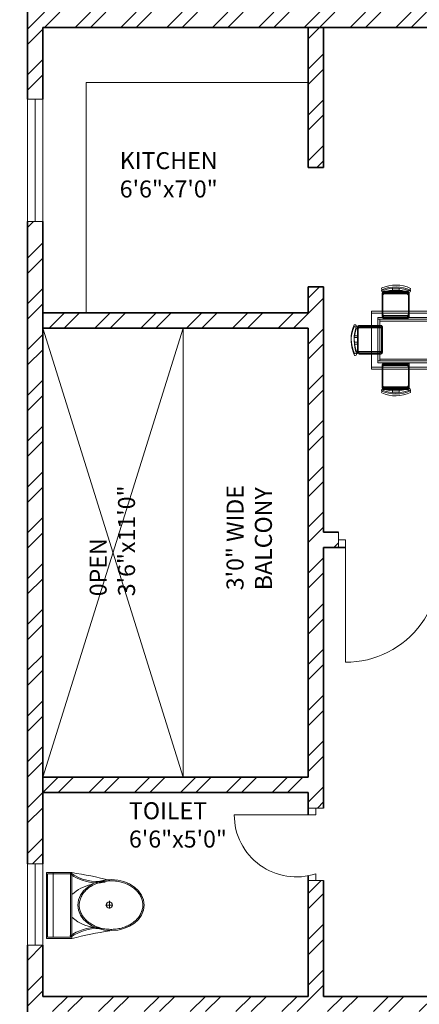
# Model space of a CAD drawing. Units: inches. Extents: x 2168 to 3056, y 1130 to 2629.
# Tile 4 of 42: x 2329 to 2447, y 1789 to 2079. Entities that reach past the tile are written whole.
import ezdxf

# ---------------------------------------------------------------- set-up
doc = ezdxf.new("R2010")
doc.units = ezdxf.units.IN
for name, color, linetype, lineweight in [('A-ANNO-DIMS', 2, 'Continuous', 18), ('A-AREA-IDEN', 7, 'Continuous', 18), ('A-DOOR', 21, 'Continuous', 18), ('A-FLOR-CASE', 71, 'Continuous', 18), ('A-FLOR-FIXT', 9, 'Continuous', 18), ('A-FLOR-OTLN', 7, 'Continuous', 18), ('A-FURN', 8, 'Continuous', 13), ('A-GLAZ', 201, 'Continuous', 18), ('A-WALL', 7, 'Continuous', 35)]:
    doc.layers.add(name, color=color, linetype=linetype, lineweight=lineweight)
doc.layers.add('A-WALL-PATT', color=143, linetype='Continuous', lineweight=13, true_color=0x7aafdf)
doc.styles.get("Standard").update_dxf_attribs({"font": 'arial.ttf'})
doc.dimstyles.get("Standard").update_dxf_attribs({"dimtxt": 0.18, "dimasz": 0.18, "dimexe": 0.18, "dimexo": 0.0625, "dimgap": 0.09, "dimtad": 0, "dimtih": 1, "dimtoh": 1, "dimdec": 4, "dimzin": 0, "dimdsep": 46, "dimtxsty": 'Standard', "dimcen": 0.09, "dimadec": 0, "dimazin": 0, "dimtfac": 1, "dimtdec": 4, "dimtofl": 0, "dimtmove": 0, "dimatfit": 3, "dimfxl": 1, "dimtolj": 1, "dimtzin": 0, "dimarcsym": 0})

# ---------------------------------------------------------------- blocks, each defined once
blk = doc.blocks.new('A$C31115884')
for p, q in [((283.1, 497.7), (223.4, 497.7)), ((257.5, 466.4), (257.5, 523.2)), ((0, 200), (0, 0)), ((520, 200), (0, 200)), ((10, 190), (10, 10)), ((510, 190), (10, 190)), ((510, 10), (510, 190)), ((520, 0), (520, 200)), ((510, 54.5), (0, 54.5)), ((10, 10), (510, 10)), ((0, 0), (520, 0))]:
    blk.add_line(p, q)
blk.add_circle((255.6, 496.4), 23.6)
for centre, radius, start, end in [((2777.7, -204.6), 2807, 165.4549, 171.71327), ((3237, 905), 2807, 188.28673, 194.5451), ((-294.5, 403.3), 364.7, 324.20913, 9.34987), ((-294.5, 403.3), 374.7, 324.20913, 9.34987), ((139.5, 406.2), 293.5, 315.84364, 2.65635), ((805.8, 403.3), 374.7, 179.20365, 215.79087), ((805.8, 403.3), 364.7, 170.65013, 215.79087), ((383.6, 406.2), 293.5, 190.27735, 224.15636)]:
    blk.add_arc(centre, radius, start, end)
blk.add_ellipse((256.2, 509.9), major_axis=(0, -260.7), ratio=0.772727)
blk.add_open_spline([(256.2, 259.2), (263.1, 259.2), (270, 259.7), (287.8, 262.3), (298.7, 265.1), (319.9, 273.1), (330.2, 278.4), (350.1, 291.1), (359.7, 298.7), (377.7, 315.9), (386.2, 325.5), (401.7, 346.6), (408.8, 358.1), (421.3, 382.5), (426.8, 395.5), (435.9, 422.4), (439.5, 436.4), (444.8, 465.1), (446.5, 479.7), (447.9, 509.2), (447.6, 524), (445, 553.3), (442.7, 567.8), (436.3, 596), (432.1, 609.7), (421.9, 636), (416, 648.6), (402.5, 672.1), (395, 683), (378.6, 703), (369.8, 712.1), (351.1, 728), (341.3, 734.8), (320.9, 746.2), (310.4, 750.7), (288.9, 757.3), (278, 759.4), (256, 761), (245, 760.6), (223.1, 757.2), (212.3, 754.3), (191.1, 746.1), (180.8, 740.7), (160.9, 727.8), (151.4, 720.1), (133.5, 702.7), (125.1, 693), (109.6, 671.7), (102.6, 660.2), (90.2, 635.7), (84.9, 622.7), (76, 595.6), (72.4, 581.6), (67.2, 552.9), (65.6, 538.2), (64.4, 508.8), (64.8, 494), (67.5, 464.7), (69.9, 450.2), (76.6, 422), (80.8, 408.3), (91.1, 382.2), (97.2, 369.7), (110.8, 346.3), (118.4, 335.4), (134.8, 315.6), (143.7, 306.7), (162.4, 290.9), (172.3, 284.2), (192.8, 273), (203.3, 268.6), (224.8, 262.2), (235.8, 260.2), (249.9, 259.3), (253, 259.2), (256.2, 259.2)], degree=3, knots=[0, 0, 0, 0, 0.110105, 0.110105, 0.285049, 0.285049, 0.459994, 0.459994, 0.634938, 0.634938, 0.809882, 0.809882, 0.984827, 0.984827, 1.159771, 1.159771, 1.334715, 1.334715, 1.50966, 1.50966, 1.684604, 1.684604, 1.859549, 1.859549, 2.034493, 2.034493, 2.209437, 2.209437, 2.384382, 2.384382, 2.559326, 2.559326, 2.73427, 2.73427, 2.909215, 2.909215, 3.084159, 3.084159, 3.259103, 3.259103, 3.434048, 3.434048, 3.608992, 3.608992, 3.783936, 3.783936, 3.958881, 3.958881, 4.133825, 4.133825, 4.30877, 4.30877, 4.483714, 4.483714, 4.658658, 4.658658, 4.833603, 4.833603, 5.008547, 5.008547, 5.183491, 5.183491, 5.358436, 5.358436, 5.53338, 5.53338, 5.708324, 5.708324, 5.883269, 5.883269, 6.058213, 6.058213, 6.233158, 6.233158, 6.283185, 6.283185, 6.283185, 6.283185])
blk = doc.blocks.new('TABLE-DINING')
for points in [[(0, 17.02), (27.45, 17.02), (27.45, 0.55), (0, 0.55)], [(0, 17.02), (27.45, 17.02), (27.45, 0.55), (0, 0.55)], [(0, 16.47), (27.45, 16.47), (27.45, 0), (0, 0)], [(0, 16.47), (27.45, 16.47), (27.45, 0), (0, 0)], [(1.83, 15.19), (25.62, 15.19), (25.62, 2.38), (1.83, 2.38)], [(1.83, 15.19), (25.62, 15.19), (25.62, 2.38), (1.83, 2.38)], [(1.83, 14.64), (25.62, 14.64), (25.62, 1.83), (1.83, 1.83)], [(1.83, 14.64), (25.62, 14.64), (25.62, 1.83), (1.83, 1.83)], [(2.38, 14.64), (25.07, 14.64), (25.07, 2.93), (2.38, 2.93)], [(2.38, 14.64), (25.07, 14.64), (25.07, 2.93), (2.38, 2.93)], [(2.38, 14.09), (25.07, 14.09), (25.07, 2.38), (2.38, 2.38)], [(2.38, 14.09), (25.07, 14.09), (25.07, 2.38), (2.38, 2.38)]]:
    blk.add_lwpolyline(points, close=True)
blk = doc.blocks.new('WIN-24')
for p, q in [((0, 0), (0, 4.5)), ((0, 4.5), (0, 2.25)), ((0, 4.5), (24, 4.5)), ((24, 2.25), (24, 4.5)), ((24, 4.5), (24, 0)), ((0, 2.25), (24, 2.25)), ((24, 0), (0, 0))]:
    blk.add_line(p, q)
blk = doc.blocks.new('WIN-36')
for p, q in [((2.25, 36), (0, 36)), ((0, 36), (4.5, 36)), ((0, 36), (0, 0)), ((2.25, 0), (2.25, 36)), ((4.5, 36), (4.5, 0)), ((0, 0), (4.5, 0)), ((4.5, 0), (2.25, 0))]:
    blk.add_line(p, q)
blk = doc.blocks.new('*D41')
at = {"layer": 'A-ANNO-DIMS', "color": 0, "lineweight": -2, "transparency": 16777216}
for p, q in [((2331.73, 2478.39), (2273.32, 2478.39)), ((2273.5, 2478.21), (2273.5, 1928.07)), ((2273.5, 1377.57), (2273.5, 1927.71)), ((2331.73, 1377.39), (2273.32, 1377.39))]:
    blk.add_line(p, q, dxfattribs=at)
at = {"layer": 'A-ANNO-DIMS', "color": 0, "transparency": 16777216}
for points in [[(2273.47, 2478.21), (2273.53, 2478.21), (2273.5, 2478.39)], [(2273.47, 1377.57), (2273.53, 1377.57), (2273.5, 1377.39)]]:
    blk.add_solid(points, dxfattribs=at)
at = {"layer": 'Defpoints', "color": 0, "transparency": 16777216}
for p in [(2273.5, 2478.39), (2331.8, 2478.39), (2331.8, 1377.39)]:
    blk.add_point(p, dxfattribs=at)
at = {"layer": 'A-ANNO-DIMS', "color": 0, "transparency": 16777216, "insert": (2273.5, 1927.89), "char_height": 0.18, "attachment_point": 5}
blk.add_mtext('\\A1;1101', dxfattribs=at)

msp = doc.modelspace()

# ---------------------------------------------------------------- hatches: boundary and pattern name
at = {"layer": 'A-WALL-PATT'}
h = msp.add_hatch(dxfattribs=at)
h.set_pattern_fill('ANSI32', color=256)
h.paths.add_polyline_path([(2463.8, 2409.39), (2467.39, 2409.39), (2467.39, 2413.89), (2454.77, 2413.89), (2454.77, 2411.64), (2454.77, 2409.39), (2459.3, 2409.39), (2459.3, 2265.39), (2455.64, 2265.39), (2455.64, 2260.89), (2467.35, 2260.89), (2467.35, 2263.14), (2467.35, 2265.39), (2463.8, 2265.39)])
h.paths.add_polyline_path([(2431.6, 2413.89), (2409.65, 2413.89), (2409.65, 2409.39), (2431.6, 2409.39), (2431.6, 2411.64)])
h.paths.add_polyline_path([(2349.65, 2413.89), (2331.8, 2413.89), (2331.8, 2362.67), (2336.3, 2362.67), (2336.3, 2409.39), (2349.65, 2409.39), (2349.65, 2411.64)])
h.paths.add_polyline_path([(2634.15, 2411.64), (2634.15, 2413.89), (2562.29, 2413.89), (2562.29, 2409.39), (2595.8, 2409.39), (2595.8, 2280.31), (2595.83, 2280.31), (2595.83, 2265.39), (2499.91, 2265.39), (2499.91, 2260.89), (2550.8, 2260.89), (2550.8, 2117.31), (2555.3, 2117.31), (2555.3, 2168.08), (2571.93, 2168.08), (2571.93, 2176.89), (2559.8, 2176.89), (2559.8, 2256.39), (2640.8, 2256.39), (2640.8, 2176.89), (2626.43, 2176.89), (2626.43, 2168.08), (2645.3, 2168.08), (2645.3, 2116.64), (2649.8, 2116.64), (2649.8, 2260.89), (2691.25, 2260.89), (2691.25, 2263.14), (2691.25, 2265.39), (2670.65, 2265.39), (2670.65, 2265.36), (2600.3, 2265.36), (2600.3, 2280.26), (2600.3, 2409.39), (2634.15, 2409.39)])
h.paths.add_polyline_path([(2600.3, 2473.89), (2612.84, 2473.89), (2612.84, 2478.39), (2572.64, 2478.39), (2572.64, 2473.89), (2595.8, 2473.89), (2595.8, 2413.89), (2600.3, 2413.89)])
h.paths.add_polyline_path([(2535.8, 2473.89), (2548.64, 2473.89), (2548.64, 2478.39), (2531.4, 2478.39), (2531.4, 2413.89), (2521.6, 2413.89), (2521.6, 2409.39), (2539.24, 2409.39), (2539.24, 2411.64), (2539.24, 2413.89), (2535.8, 2413.89)])
h.paths.add_polyline_path([(2664.8, 2478.39), (2636.84, 2478.39), (2636.84, 2473.89), (2660.3, 2473.89), (2660.3, 2413.89), (2656.17, 2413.89), (2656.17, 2409.39), (2671.68, 2409.39), (2671.68, 2411.64), (2671.68, 2413.89), (2664.8, 2413.89)])
h.paths.add_polyline_path([(2705.94, 2413.89), (2695.68, 2413.89), (2695.68, 2409.39), (2705.94, 2409.39)])
h.paths.add_polyline_path([(2741.35, 2413.89), (2728.73, 2413.89), (2728.73, 2411.64), (2728.73, 2409.39), (2732.3, 2409.39), (2732.3, 2265.39), (2725.73, 2265.39), (2725.73, 2260.89), (2740.92, 2260.89), (2740.92, 2263.14), (2740.92, 2265.39), (2736.8, 2265.39), (2736.8, 2409.39), (2741.35, 2409.39)])
h.paths.add_polyline_path([(2785.65, 2413.89), (2764.55, 2413.89), (2764.49, 2409.39), (2785.65, 2409.39), (2785.65, 2411.64)])
h.paths.add_polyline_path([(2864.3, 2413.89), (2845.65, 2413.89), (2845.65, 2409.39), (2859.8, 2409.39), (2859.8, 2368.43), (2864.3, 2368.43)])
h.paths.add_polyline_path([(2864.3, 2308.43), (2862.05, 2308.43), (2859.8, 2308.43), (2859.8, 2265.39), (2774.48, 2265.39), (2774.48, 2263.14), (2774.48, 2260.89), (2781.8, 2260.89), (2781.8, 2226.65), (2786.3, 2226.65), (2786.3, 2260.89), (2859.8, 2260.89), (2859.8, 2241.35), (2864.3, 2241.35)])
h.paths.add_polyline_path([(2864.3, 2217.35), (2862.05, 2217.35), (2859.8, 2217.35), (2859.8, 2200.89), (2786.3, 2200.89), (2786.3, 2205.93), (2784.05, 2205.93), (2781.8, 2205.93), (2781.8, 2150.97), (2786.3, 2150.97), (2786.3, 2161.89), (2859.8, 2161.89), (2859.8, 2144.42), (2864.3, 2144.42)])
h.paths.add_polyline_path([(2859.8, 2196.39), (2859.8, 2166.39), (2786.3, 2166.39), (2786.3, 2196.39)], flags=16)
h.paths.add_polyline_path([(2864.3, 2108.42), (2862.05, 2108.42), (2859.8, 2108.42), (2859.8, 2080.89), (2786.3, 2080.89), (2786.3, 2111.99), (2781.8, 2111.99), (2781.8, 2080.89), (2649.8, 2080.89), (2649.8, 2086.04), (2647.55, 2086.04), (2645.3, 2086.04), (2645.3, 2071.74), (2649.8, 2071.74), (2649.8, 2076.39), (2781.8, 2076.39), (2781.8, 2041.79), (2786.3, 2041.79), (2786.3, 2076.39), (2859.8, 2076.39), (2859.8, 2058.58), (2864.3, 2058.58)])
h.paths.add_polyline_path([(2864.3, 2022.58), (2859.8, 2022.58), (2859.8, 1992.39), (2786.3, 1992.39), (2786.3, 1999.57), (2781.8, 1999.57), (2781.8, 1848.09), (2784.05, 1848.09), (2786.3, 1848.09), (2786.3, 1851.39), (2859.8, 1851.39), (2859.8, 1838.26), (2864.3, 1838.26)], flags=17)
h.paths.add_polyline_path([(2859.8, 1987.89), (2859.8, 1855.89), (2786.3, 1855.89), (2786.3, 1987.89)], flags=16)
h.paths.add_polyline_path([(2823.05, 1987.89), (2841.42, 1921.89), (2823.05, 1855.89)], flags=0)
h.paths.add_polyline_path([(2864.3, 1814.26), (2859.8, 1814.26), (2859.8, 1791.39), (2786.3, 1791.39), (2786.3, 1825.66), (2784.05, 1825.66), (2781.8, 1825.66), (2781.8, 1791.39), (2720.15, 1791.39), (2720.15, 1791.27), (2649.8, 1791.27), (2649.8, 1806.16), (2649.8, 2038.98), (2647.55, 2038.98), (2645.3, 2038.98), (2645.3, 1783.93), (2649.8, 1783.93), (2649.8, 1786.89), (2781.8, 1786.89), (2781.8, 1746.79), (2786.3, 1746.79), (2786.3, 1786.89), (2859.8, 1786.89), (2859.8, 1770.08), (2864.3, 1770.08)])
h.paths.add_polyline_path([(2864.3, 1734.08), (2862.05, 1734.08), (2859.8, 1734.08), (2859.8, 1705.89), (2786.3, 1705.89), (2786.3, 1714.17), (2781.8, 1714.17), (2781.8, 1660.53), (2786.3, 1660.53), (2786.3, 1666.89), (2859.8, 1666.89), (2859.8, 1648.34), (2864.3, 1648.34)])
h.paths.add_polyline_path([(2786.3, 1701.39), (2859.8, 1701.39), (2859.8, 1671.39), (2786.3, 1671.39)], flags=16)
h.paths.add_polyline_path([(2649.8, 1756.58), (2647.55, 1756.58), (2645.3, 1756.58), (2645.3, 1606.89), (2555.3, 1606.89), (2555.3, 1749.51), (2553.05, 1749.51), (2550.8, 1749.51), (2550.8, 1606.89), (2503.01, 1606.89), (2503.01, 1604.64), (2503.01, 1602.39), (2595.8, 1602.39), (2595.85, 1602.39), (2595.85, 1587.5), (2595.8, 1458.39), (2561.5, 1458.39), (2561.5, 1456.14), (2561.5, 1453.89), (2595.8, 1453.89), (2595.8, 1381.89), (2573.44, 1381.89), (2573.44, 1377.39), (2613.01, 1377.39), (2613.01, 1379.64), (2613.01, 1381.89), (2600.3, 1381.89), (2600.3, 1453.89), (2634.33, 1453.89), (2634.33, 1458.39), (2600.3, 1458.39), (2600.3, 1602.39), (2670.65, 1602.39), (2694.09, 1602.39), (2694.09, 1606.89), (2649.8, 1606.89)])
h.paths.add_polyline_path([(2736.8, 1602.39), (2741.56, 1602.39), (2741.56, 1606.89), (2726.2, 1606.89), (2726.2, 1604.64), (2726.2, 1602.39), (2732.3, 1602.39), (2732.3, 1458.39), (2727.9, 1458.39), (2727.9, 1453.89), (2740.82, 1453.89), (2740.82, 1456.14), (2740.82, 1458.39), (2736.8, 1458.39)])
h.paths.add_polyline_path([(2859.8, 1606.89), (2786.3, 1606.89), (2786.3, 1637.33), (2784.05, 1637.33), (2781.8, 1637.33), (2781.8, 1606.89), (2775.61, 1606.89), (2775.61, 1602.39), (2859.8, 1602.39)])
h.paths.add_polyline_path([(2864.3, 1624.34), (2862.05, 1624.34), (2859.8, 1624.34), (2859.8, 1570.39), (2864.3, 1570.39)])
h.paths.add_polyline_path([(2864.3, 1510.39), (2862.05, 1510.39), (2859.8, 1510.39), (2859.8, 1458.39), (2846.73, 1458.39), (2846.73, 1456.14), (2846.73, 1453.89), (2864.3, 1453.89)])
h.paths.add_polyline_path([(2786.73, 1458.39), (2765.44, 1458.39), (2765.44, 1453.89), (2786.73, 1453.89)])
h.paths.add_polyline_path([(2706, 1458.39), (2695.36, 1458.39), (2695.36, 1453.89), (2706, 1453.89), (2706, 1456.14)])
h.paths.add_polyline_path([(2671.36, 1456.14), (2671.36, 1458.39), (2655.99, 1458.39), (2655.99, 1456.14), (2655.99, 1453.89), (2660.3, 1453.89), (2660.3, 1381.89), (2637.01, 1381.89), (2637.01, 1377.39), (2664.8, 1377.39), (2664.8, 1453.89), (2671.36, 1453.89)], flags=17)
h.paths.add_polyline_path([(2539.83, 1458.39), (2520.24, 1458.39), (2520.24, 1453.89), (2531.3, 1453.89), (2531.3, 1377.39), (2546.45, 1377.39), (2546.45, 1379.64), (2546.45, 1381.89), (2535.8, 1381.89), (2535.8, 1453.89), (2539.83, 1453.89)], flags=17)
h.paths.add_polyline_path([(2496.24, 1458.39), (2489.13, 1458.39), (2489.13, 1453.89), (2496.24, 1453.89), (2496.24, 1456.14)])
h.paths.add_polyline_path([(2467.43, 1456.14), (2467.43, 1458.39), (2463.8, 1458.39), (2463.8, 1602.39), (2468.24, 1602.39), (2468.24, 1605.7), (2468.24, 1606.89), (2454.6, 1606.89), (2454.6, 1602.39), (2459.3, 1602.39), (2459.3, 1458.39), (2454.24, 1458.39), (2454.24, 1453.89), (2467.43, 1453.89)])
h.paths.add_polyline_path([(2431.6, 1456.14), (2431.6, 1458.39), (2411.39, 1458.39), (2411.39, 1453.89), (2431.6, 1453.89)])
h.paths.add_polyline_path([(2351.39, 1458.39), (2336.3, 1458.39), (2336.3, 1490.69), (2334.05, 1490.69), (2331.8, 1490.69), (2331.8, 1453.89), (2351.39, 1453.89), (2351.39, 1456.14)])
h.paths.add_polyline_path([(2336.3, 1629.7), (2331.8, 1629.7), (2331.8, 1552.32), (2336.3, 1552.32), (2336.3, 1602.39), (2406.65, 1602.39), (2423.47, 1602.39), (2423.47, 1606.89), (2418.8, 1606.89), (2418.8, 1643.68), (2416.55, 1643.68), (2414.3, 1643.68), (2414.3, 1606.89), (2336.3, 1606.89)])
h.paths.add_polyline_path([(2418.8, 1714.38), (2414.3, 1714.38), (2414.3, 1705.89), (2336.3, 1705.89), (2336.3, 1731.32), (2334.05, 1731.32), (2331.8, 1731.32), (2331.8, 1653.7), (2334.05, 1653.7), (2336.3, 1653.7), (2336.3, 1666.89), (2414.3, 1666.89), (2414.3, 1663.59), (2418.8, 1663.59)])
h.paths.add_polyline_path([(2336.3, 1701.39), (2414.3, 1701.39), (2414.3, 1671.39), (2336.3, 1671.39)], flags=16)
h.paths.add_polyline_path([(2555.3, 2040.06), (2550.8, 2040.06), (2550.8, 1791.39), (2550.56, 1791.2), (2480.2, 1791.2), (2418.8, 1791.39), (2418.8, 1825.45), (2416.55, 1825.45), (2414.3, 1825.45), (2414.3, 1791.39), (2336.3, 1791.39), (2336.3, 1806.41), (2331.8, 1806.41), (2331.8, 1767.32), (2336.3, 1767.32), (2336.3, 1786.89), (2414.3, 1786.89), (2414.3, 1745.46), (2418.8, 1745.46), (2418.8, 1786.89), (2550.8, 1786.89), (2550.8, 1783.01), (2555.3, 1783.01)])
h.paths.add_polyline_path([(2418.8, 1923.39), (2423.21, 1923.39), (2423.21, 1925.64), (2423.21, 1927.89), (2418.8, 1927.89), (2418.8, 2000.05), (2414.3, 2000.05), (2414.3, 1992.39), (2336.3, 1992.39), (2336.3, 1987.89), (2414.3, 1987.89), (2414.3, 1855.89), (2336.3, 1855.89), (2336.3, 1851.39), (2414.3, 1851.39), (2414.3, 1846.76), (2418.8, 1846.76)], flags=17)
h.paths.add_polyline_path([(2336.3, 2019.29), (2334.05, 2019.29), (2331.8, 2019.29), (2331.8, 1830.41), (2336.3, 1830.41)], flags=17)
h.paths.add_polyline_path([(2550.8, 1927.89), (2453.54, 1927.89), (2453.54, 1925.64), (2453.54, 1923.39), (2550.8, 1923.39)], flags=17)
h.paths.add_polyline_path([(2744.99, 1927.89), (2649.8, 1927.89), (2649.8, 1923.39), (2744.99, 1923.39), (2744.99, 1925.64)], flags=17)
h.paths.add_polyline_path([(2555.3, 2086.46), (2553.05, 2086.46), (2550.8, 2086.46), (2550.8, 2080.89), (2418.8, 2080.89), (2336.3, 2080.89), (2336.3, 2115.4), (2334.05, 2115.4), (2331.8, 2115.4), (2331.8, 2055.29), (2336.3, 2055.29), (2336.3, 2076.39), (2550.8, 2076.39), (2550.8, 2071.54), (2555.3, 2071.54)])
h.paths.add_polyline_path([(2418.8, 2121.39), (2414.3, 2121.39), (2414.3, 2080.89), (2418.8, 2080.89)])
h.paths.add_polyline_path([(2418.8, 2076.39), (2414.3, 2076.39), (2414.3, 2035.12), (2418.8, 2035.12)])
h.paths.add_polyline_path([(2422.87, 2263.14), (2422.87, 2265.39), (2406.65, 2265.39), (2406.65, 2265.36), (2336.3, 2265.36), (2336.3, 2280.25), (2336.3, 2302.67), (2334.05, 2302.67), (2331.8, 2302.67), (2331.8, 2246.85), (2336.3, 2246.85), (2336.3, 2260.89), (2414.3, 2260.89), (2414.3, 2224), (2418.8, 2224), (2418.8, 2260.89), (2422.87, 2260.89)])
h.paths.add_polyline_path([(2418.8, 2204.78), (2416.55, 2204.78), (2414.3, 2204.78), (2414.3, 2200.89), (2336.3, 2200.89), (2336.3, 2220.85), (2331.8, 2220.85), (2331.8, 2151.4), (2336.3, 2151.4), (2336.3, 2161.89), (2414.3, 2161.89), (2414.3, 2153.73), (2418.8, 2153.73)])
h.paths.add_polyline_path([(2414.3, 2196.39), (2414.3, 2166.39), (2336.3, 2166.39), (2336.3, 2196.39)], flags=16)
h.paths.add_polyline_path([(2375.3, 2181.39), (2336.3, 2166.39), (2336.3, 2196.39)], flags=0)
h.paths.add_polyline_path([(2809.6, 2172.34), (2838.8, 2172.34), (2838.8, 2191), (2809.6, 2191)], flags=8)
h.paths.add_polyline_path([(2849.75, 1919.59), (2849.75, 1952.67), (2831.09, 1952.67), (2831.09, 1919.59)], flags=8)
h.paths.add_polyline_path([(2808.87, 1901.97), (2808.87, 1937.85), (2790.15, 1937.85), (2790.15, 1901.97)], flags=8)
h.paths.add_polyline_path([(2806.28, 1671.9), (2835.49, 1671.9), (2835.49, 1690.55), (2806.28, 1690.55)], flags=8)
h.paths.add_polyline_path([(2353.19, 1676.55), (2382.39, 1676.55), (2382.39, 1695.21), (2353.19, 1695.21)], flags=8)
h.paths.add_polyline_path([(2360.08, 1832.31), (2389.24, 1832.31), (2389.24, 1850.97), (2360.08, 1850.97)], flags=25)
h.paths.add_polyline_path([(2354.82, 2167.82), (2384.03, 2167.82), (2384.03, 2186.48), (2354.82, 2186.48)], flags=8)

# ---------------------------------------------------------------- linework, layer by layer
at = {"layer": 'A-DOOR'}
for p, q in [((2423.21, 1927.89), (2423.21, 1923.39)), ((2423.21, 1923.39), (2423.21, 1925.64)), ((2423.21, 1925.64), (2425.21, 1925.64)), ((2425.21, 1925.64), (2425.21, 1889.64)), ((2416.55, 1844.76), (2392.55, 1844.76)), ((2414.3, 1846.76), (2418.8, 1846.76)), ((2418.8, 1846.76), (2416.55, 1846.76)), ((2416.55, 1846.76), (2416.55, 1844.76)), ((2416.55, 1825.45), (2416.55, 1827.45)), ((2414.3, 1825.45), (2418.8, 1825.45)), ((2418.8, 1825.45), (2416.55, 1825.45))]:
    msp.add_line(p, q, dxfattribs=at)
for centre, radius, start, end in [((2425.21, 1917.27), 27.63, 270, 17.6272), ((2410.79, 1844.76), 18.24, 180, 288.3963)]:
    msp.add_arc(centre, radius, start, end, dxfattribs=at)
at = {"layer": 'A-FLOR-CASE'}
for p, q in [((2414.3, 2060.13), (2349, 2060.13)), ((2349, 2060.13), (2349, 1992.39))]:
    msp.add_line(p, q, dxfattribs=at)
at = {"layer": 'A-FLOR-OTLN'}
for p, q in [((2377.55, 1987.89), (2336.3, 1855.89)), ((2336.3, 1987.89), (2377.55, 1855.89)), ((2377.55, 1855.89), (2377.55, 1987.89))]:
    msp.add_line(p, q, dxfattribs=at)
at = {"layer": 'A-FURN'}
for points in [[(2436.32, 1999.05, -0.175809), (2443.79, 1999, 0.578392), (2444.36, 1999.62, 0.214524), (2435.92, 1999.73, 0.552014), (2436.32, 1999.05, -0.065079)], [(2436.32, 1999.05, -0.175809), (2443.79, 1999, 0.578392), (2444.36, 1999.62, 0.214524), (2435.92, 1999.73, 0.552014), (2436.32, 1999.05, -0.065079)], [(2436.32, 1998.51, -0.175809), (2443.79, 1998.45, 0.578392), (2444.36, 1999.07, 0.214524), (2435.92, 1999.18, 0.552014), (2436.32, 1998.51, -0.065079)], [(2436.32, 1998.5, -0.175809), (2443.79, 1998.45, 0.578392), (2444.36, 1999.07, 0.214524), (2435.92, 1999.18, 0.552014), (2436.32, 1998.5, -0.065079)], [(2443.47, 1998.75), (2436.53, 1998.75, 0.414214), (2436.05, 1998.27), (2436.05, 1991.89, 0.414214), (2436.53, 1991.4), (2443.47, 1991.4, 0.414214), (2443.96, 1991.89), (2443.96, 1998.27, 0.414214), (2443.47, 1998.75)], [(2443.47, 1998.75), (2436.53, 1998.75, 0.414214), (2436.05, 1998.27), (2436.05, 1991.89, 0.414214), (2436.53, 1991.4), (2443.47, 1991.4, 0.414214), (2443.96, 1991.89), (2443.96, 1998.27, 0.414214), (2443.47, 1998.75)], [(2443.47, 1998.21), (2436.53, 1998.21, 0.414214), (2436.05, 1997.72), (2436.05, 1991.34, 0.414214), (2436.53, 1990.85), (2443.47, 1990.85, 0.414214), (2443.96, 1991.34), (2443.96, 1997.72, 0.414214), (2443.47, 1998.21)], [(2443.47, 1998.2), (2436.53, 1998.2, 0.414214), (2436.05, 1997.72), (2436.05, 1991.34, 0.414214), (2436.53, 1990.85), (2443.47, 1990.85, 0.414214), (2443.96, 1991.34), (2443.96, 1997.72, 0.414214), (2443.47, 1998.2)], [(2441.04, 1998.75), (2441.04, 1999.63, -0.064759)], [(2441.04, 1998.75), (2441.04, 1999.63, -0.064759)], [(2441.04, 1998.21), (2441.04, 1999.08, -0.064759)], [(2441.04, 1998.2), (2441.04, 1999.08, -0.064759)], [(2428.5, 1981, -0.578392), (2427.87, 1980.44, -0.214524), (2427.76, 1988.87, -0.552014), (2428.44, 1988.48, 0.175809), (2428.5, 1981)], [(2428.5, 1981, -0.578392), (2427.87, 1980.44, -0.214524), (2427.76, 1988.87, -0.552014), (2428.44, 1988.48, 0.175809), (2428.5, 1981)], [(2428.5, 1980.45, -0.578392), (2427.87, 1979.89, -0.214524), (2427.76, 1988.33, -0.552014), (2428.44, 1987.93, 0.175809), (2428.5, 1980.45)], [(2428.5, 1980.45, -0.578392), (2427.87, 1979.89, -0.214524), (2427.76, 1988.32, -0.552014), (2428.44, 1987.93, 0.175809), (2428.5, 1980.45)], [(2428.74, 1988.26, -0.414214), (2429.22, 1988.74), (2435.61, 1988.74, -0.414214), (2436.09, 1988.26), (2436.09, 1981.32, -0.414214), (2435.61, 1980.83), (2429.22, 1980.83, -0.414214), (2428.74, 1981.32), (2428.74, 1988.26)], [(2428.74, 1988.26, -0.414214), (2429.22, 1988.74), (2435.61, 1988.74, -0.414214), (2436.09, 1988.26), (2436.09, 1981.32, -0.414214), (2435.61, 1980.83), (2429.22, 1980.83, -0.414214), (2428.74, 1981.32), (2428.74, 1988.26)], [(2428.74, 1987.71, -0.414214), (2429.22, 1988.2), (2435.61, 1988.2, -0.414214), (2436.09, 1987.71), (2436.09, 1980.77, -0.414214), (2435.61, 1980.28), (2429.22, 1980.28, -0.414214), (2428.74, 1980.77), (2428.74, 1987.71)], [(2428.74, 1987.71, -0.414214), (2429.22, 1988.2), (2435.61, 1988.2, -0.414214), (2436.09, 1987.71), (2436.09, 1980.77, -0.414214), (2435.61, 1980.28), (2429.22, 1980.28, -0.414214), (2428.74, 1980.77), (2428.74, 1987.71)], [(2428.74, 1983.76), (2427.86, 1983.76, 0.064759)], [(2428.74, 1983.76), (2427.86, 1983.76, 0.064759)], [(2428.74, 1983.21), (2427.86, 1983.21, 0.064759)], [(2428.74, 1983.21), (2427.86, 1983.21, 0.064759)], [(2443.47, 1970.39), (2436.53, 1970.39, -0.414214), (2436.05, 1970.87), (2436.05, 1977.26, -0.414214), (2436.53, 1977.74), (2443.47, 1977.74, -0.414214), (2443.96, 1977.26), (2443.96, 1970.87, -0.414214), (2443.47, 1970.39)], [(2443.47, 1970.39), (2436.53, 1970.39, -0.414214), (2436.05, 1970.87), (2436.05, 1977.25, -0.414214), (2436.53, 1977.74), (2443.47, 1977.74, -0.414214), (2443.96, 1977.25), (2443.96, 1970.87, -0.414214), (2443.47, 1970.39)], [(2443.47, 1969.84), (2436.53, 1969.84, -0.414214), (2436.05, 1970.33), (2436.05, 1976.71, -0.414214), (2436.53, 1977.19), (2443.47, 1977.19, -0.414214), (2443.96, 1976.71), (2443.96, 1970.33, -0.414214), (2443.47, 1969.84)], [(2443.47, 1969.84), (2436.53, 1969.84, -0.414214), (2436.05, 1970.32), (2436.05, 1976.71, -0.414214), (2436.53, 1977.19), (2443.47, 1977.19, -0.414214), (2443.96, 1976.71), (2443.96, 1970.32, -0.414214), (2443.47, 1969.84)], [(2443.79, 1970.14, -0.578392), (2444.36, 1969.52, -0.214524), (2435.92, 1969.41, -0.552014), (2436.32, 1970.09, 0.175809), (2443.79, 1970.14)], [(2443.79, 1970.14, -0.578392), (2444.36, 1969.52, -0.214524), (2435.92, 1969.41, -0.552014), (2436.32, 1970.09, 0.175809), (2443.79, 1970.14)], [(2443.79, 1969.6, -0.578392), (2444.36, 1968.97, -0.214524), (2435.92, 1968.86, -0.552014), (2436.32, 1969.54, 0.175809), (2443.79, 1969.6)], [(2443.79, 1969.6, -0.578392), (2444.36, 1968.97, -0.214524), (2435.92, 1968.86, -0.552014), (2436.32, 1969.54, 0.175809), (2443.79, 1969.6)], [(2441.04, 1970.39), (2441.04, 1969.51, 0.064759)], [(2441.04, 1970.39), (2441.04, 1969.51, 0.064759)], [(2441.04, 1969.84), (2441.04, 1968.96, 0.064759)], [(2441.04, 1969.84), (2441.04, 1968.96, 0.064759)]]:
    msp.add_lwpolyline(points, format="xyb", dxfattribs=at)
for points in [[(2436.54, 1998.54), (2443.26, 1998.54, -0.414214), (2443.74, 1998.05), (2443.74, 1992.11, -0.414214), (2443.26, 1991.62), (2436.54, 1991.62, -0.512069), (2436.27, 1992.11), (2436.27, 1998.05, -0.512069)], [(2436.54, 1998.54), (2443.26, 1998.54, -0.414214), (2443.74, 1998.05), (2443.74, 1992.11, -0.414214), (2443.26, 1991.62), (2436.54, 1991.62, -0.512069), (2436.27, 1992.11), (2436.27, 1998.05, -0.512069)], [(2436.54, 1997.99), (2443.26, 1997.99, -0.414214), (2443.74, 1997.5), (2443.74, 1991.56, -0.414214), (2443.26, 1991.07), (2436.54, 1991.07, -0.512069), (2436.27, 1991.56), (2436.27, 1997.5, -0.512069)], [(2436.54, 1997.99), (2443.26, 1997.99, -0.414214), (2443.74, 1997.5), (2443.74, 1991.56, -0.414214), (2443.26, 1991.07), (2436.54, 1991.07, -0.512069), (2436.27, 1991.56), (2436.27, 1997.5, -0.512069)], [(2428.96, 1988.26), (2428.96, 1981.54, 0.414214), (2429.44, 1981.05), (2435.39, 1981.05, 0.414214), (2435.87, 1981.54), (2435.87, 1988.26, 0.512069), (2435.39, 1988.53), (2429.44, 1988.53, 0.512069)], [(2428.96, 1988.26), (2428.96, 1981.54, 0.414214), (2429.44, 1981.05), (2435.39, 1981.05, 0.414214), (2435.87, 1981.54), (2435.87, 1988.26, 0.512069), (2435.39, 1988.53), (2429.44, 1988.53, 0.512069)], [(2428.96, 1987.71), (2428.96, 1980.99, 0.414214), (2429.44, 1980.5), (2435.39, 1980.5, 0.414214), (2435.87, 1980.99), (2435.87, 1987.71, 0.512069), (2435.39, 1987.98), (2429.44, 1987.98, 0.512069)], [(2428.96, 1987.71), (2428.96, 1980.99, 0.414214), (2429.44, 1980.5), (2435.39, 1980.5, 0.414214), (2435.87, 1980.99), (2435.87, 1987.71, 0.512069), (2435.39, 1987.98), (2429.44, 1987.98, 0.512069)], [(2436.54, 1970.61), (2443.26, 1970.61, 0.414214), (2443.74, 1971.09), (2443.74, 1977.04, 0.414214), (2443.26, 1977.52), (2436.54, 1977.52, 0.512069), (2436.27, 1977.04), (2436.27, 1971.09, 0.512069)], [(2436.54, 1970.61), (2443.26, 1970.61, 0.414214), (2443.74, 1971.09), (2443.74, 1977.04, 0.414214), (2443.26, 1977.52), (2436.54, 1977.52, 0.512069), (2436.27, 1977.04), (2436.27, 1971.09, 0.512069)], [(2436.54, 1970.06), (2443.26, 1970.06, 0.414214), (2443.74, 1970.54), (2443.74, 1976.49, 0.414214), (2443.26, 1976.97), (2436.54, 1976.97, 0.512069), (2436.27, 1976.49), (2436.27, 1970.54, 0.512069)], [(2436.54, 1970.06), (2443.26, 1970.06, 0.414214), (2443.74, 1970.54), (2443.74, 1976.49, 0.414214), (2443.26, 1976.97), (2436.54, 1976.97, 0.512069), (2436.27, 1976.49), (2436.27, 1970.54, 0.512069)]]:
    msp.add_lwpolyline(points, format="xyb", close=True, dxfattribs=at)
for points in [[(2439.09, 1999.65), (2439.09, 1998.75)], [(2439.09, 1999.65), (2439.09, 1998.75)], [(2439.09, 1999.1), (2439.09, 1998.21)], [(2439.09, 1999.1), (2439.09, 1998.2)], [(2427.85, 1985.7), (2428.74, 1985.7)], [(2427.85, 1985.7), (2428.74, 1985.7)], [(2427.85, 1985.15), (2428.74, 1985.15)], [(2427.85, 1985.15), (2428.74, 1985.15)], [(2439.09, 1969.49), (2439.09, 1970.39)], [(2439.09, 1969.49), (2439.09, 1970.39)], [(2439.09, 1968.95), (2439.09, 1969.84)], [(2439.09, 1968.95), (2439.09, 1969.84)]]:
    msp.add_lwpolyline(points, dxfattribs=at)
at = {"layer": 'A-WALL'}
for p, q in [((2331.8, 2115.4), (2331.8, 2055.29)), ((2336.3, 2076.39), (2550.8, 2076.39)), ((2336.3, 2076.39), (2336.3, 2055.29)), ((2414.3, 2076.39), (2414.3, 2035.12)), ((2418.8, 2076.39), (2418.8, 2035.12)), ((2414.3, 2035.12), (2418.8, 2035.12)), ((2331.8, 2019.29), (2331.8, 1830.41)), ((2336.3, 2019.29), (2336.3, 1830.41)), ((2414.3, 2000.05), (2418.8, 2000.05)), ((2414.3, 2000.05), (2414.3, 1992.39)), ((2418.8, 2000.05), (2418.8, 1927.89)), ((2336.3, 1992.39), (2414.3, 1992.39)), ((2336.3, 1987.89), (2414.3, 1987.89)), ((2414.3, 1987.89), (2414.3, 1855.89)), ((2418.8, 1927.89), (2423.21, 1927.89)), ((2418.8, 1923.39), (2418.8, 1846.76)), ((2425.21, 1923.39), (2418.8, 1923.39)), ((2336.3, 1855.89), (2414.3, 1855.89)), ((2336.3, 1851.39), (2414.3, 1851.39)), ((2414.3, 1851.39), (2414.3, 1844.76)), ((2414.3, 1826.86), (2414.3, 1791.39)), ((2418.8, 1825.45), (2418.8, 1791.39)), ((2331.8, 1806.41), (2331.8, 1767.32)), ((2336.3, 1806.41), (2336.3, 1791.39)), ((2336.3, 1791.39), (2414.3, 1791.39)), ((2418.8, 1791.39), (2550.8, 1791.39))]:
    msp.add_line(p, q, dxfattribs=at)

# ---------------------------------------------------------------- block references
at = {"layer": 'A-FLOR-FIXT', "xscale": 0.0372717239612423, "yscale": 0.0372717239612423, "zscale": 0.0372717239612423, "rotation": 270}
msp.add_blockref('A$C31115884', (2337.34, 1827.77), dxfattribs=at)
at = {"layer": 'A-FURN'}
msp.add_blockref('TABLE-DINING', (2432.92, 1975.88), dxfattribs=at)
at = {"layer": 'A-GLAZ'}
for name, p, rotation in [('WIN-36', (2336.3, 2055.29), 180), ('WIN-24', (2336.3, 1806.41), 90)]:
    msp.add_blockref(name, p, dxfattribs=dict(at, rotation=rotation))

# ---------------------------------------------------------------- texts
at = {"layer": 'A-AREA-IDEN', "char_height": 5, "attachment_point": 1}
for s, width, insert in [('KITCHEN\\P6\'6"x7\'0"', 209.2297, (2358.89, 2039.68)), ('TOILET\\P6\'6"x5\'0"', 205.4097, (2361.6, 1848.48))]:
    msp.add_mtext_dynamic_manual_height_columns(s, width=width, gutter_width=12.5, heights=[0], dxfattribs=dict(at, insert=insert))
at = {"layer": 'A-AREA-IDEN', "char_height": 5, "attachment_point": 1, "rotation": 90}
for s, width, insert in [('0PEN\\P3\'6"x11\'0"', 78.2938, (2350.06, 1909.06)), ('3\'0" WIDE\\PBALCONY', 123.3316, (2390.29, 1910.83))]:
    msp.add_mtext_dynamic_manual_height_columns(s, width=width, gutter_width=12.5, heights=[0], dxfattribs=dict(at, insert=insert))

# ---------------------------------------------------------------- dimensions: what is measured, and where the dimension line sits
at = {"layer": 'A-ANNO-DIMS'}
dim = msp.add_linear_dim(base=(2273.5, 2478.39), p1=(2331.8, 1377.39), p2=(2331.8, 2478.39), angle=90, dimstyle='Standard', override={"dimdec": 0, "dimlfac": 1, "dimrnd": 0, "dimzin": 0, "dimdsep": 46, "dimlunit": 2}, dxfattribs=at)
dim.commit()
dim.dimension.update_dxf_attribs({"geometry": '*D41', "text_midpoint": (2273.5, 1927.89)})

doc.saveas('drawing.dxf')
